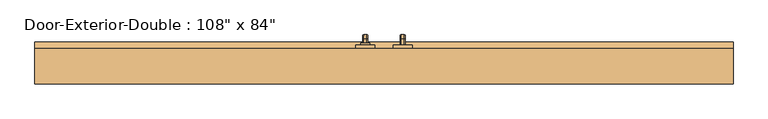
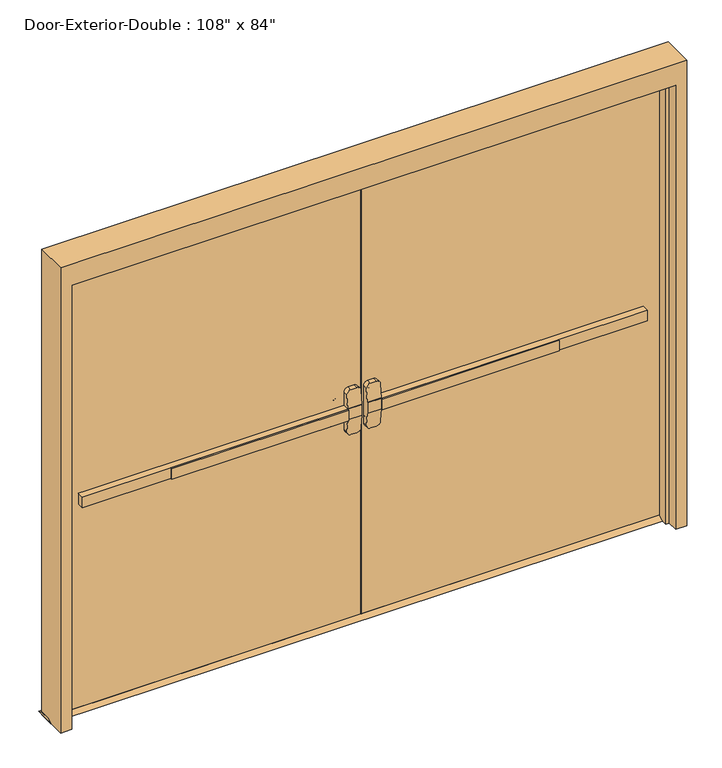
"""IFC4 building model written with IfcOpenShell, lengths in millimetres: door geometry."""

from ifc_helpers import new_model, si_unit, point, frame, frame_2d, origin, place, context, project, spatial, polyline, circle_curve, ellipse_curve, trimmed, segment, composite_curve, outline, extrude, faceted_brep, source, transform, mapped, element, save
from ifc_brep_helpers import plane_surface, cylinder_surface, revolved_surface, advanced_brep


def door_b5c84c7e(model_context):
    return source(origin(), model_context, "Body", "SolidModel", [
        extrude(outline(polyline([(-880.5333333, 0.0), (-880.5333333, 6.35), (-76.2, 6.35), (-76.2, 0.0), (-880.5333333, 0.0)])), frame((0.0, 0.0, 990.6), z_axis=(0.0, 0.0, 1.0), x_axis=(1.0, 0.0, 0.0)), (0.0, 0.0, 1.0), 50.8),
        advanced_brep(
        [(-12.7, 6.35, 1041.4), (-76.2, 6.35, 1041.4), (-1282.7, 6.35, 1041.4), (-1282.7, 6.35, 990.6), (-76.2, 6.35, 990.6), (-12.7, 6.35, 990.6), (-1282.7, 38.1, 1041.4), (-76.2, 38.1, 1041.4), (-76.2, 38.1, 1104.9), (-57.15, 38.1, 1123.95), (-31.75, 38.1, 1123.95), (-12.7, 38.1, 1104.9), (-12.7, 38.1, 927.1), (-31.75, 38.1, 908.05), (-57.15, 38.1, 908.05), (-76.2, 38.1, 927.1), (-76.2, 38.1, 990.6), (-1282.7, 38.1, 990.6), (-12.7, 9.5252467, 1041.4), (-76.2, 9.5252467, 1041.4), (-12.7, 9.5252467, 990.6), (-12.7, 14.5354269, 927.1), (-12.7, 14.5354269, 1104.9), (-76.2, 9.5252467, 990.6), (-76.2, 14.5354269, 1104.9), (-76.2, 14.5354269, 927.1), (-57.15, 16.038481, 1123.95), (-31.75, 16.038481, 1123.95), (-31.75, 16.038481, 908.05), (-57.15, 16.038481, 908.05)],
        [
            (0, 1),
            (1, 2),
            (2, 3),
            (3, 4),
            (4, 5),
            (5, 0),
            (6, 7),
            (7, 8),
            (8, 9, circle_curve(frame((-57.15, 38.1, 1104.9), z_axis=(0.0, 1.0, 0.0), x_axis=(-1.0, 0.0, 0.0)), 19.05)),
            (9, 10),
            (10, 11, circle_curve(frame((-31.75, 38.1, 1104.9), z_axis=(0.0, 1.0, 0.0), x_axis=(-1.0, 0.0, 0.0)), 19.05)),
            (11, 12),
            (12, 13, circle_curve(frame((-31.75, 38.1, 927.1), z_axis=(0.0, 1.0, 0.0), x_axis=(-1.0, 0.0, 0.0)), 19.05)),
            (13, 14),
            (14, 15, circle_curve(frame((-57.15, 38.1, 927.1), z_axis=(0.0, 1.0, 0.0), x_axis=(-1.0, 0.0, 0.0)), 19.05)),
            (15, 16),
            (16, 17),
            (17, 6),
            (0, 18),
            (18, 19),
            (19, 7),
            (6, 2),
            (5, 20),
            (20, 21),
            (21, 12),
            (11, 22),
            (22, 18),
            (16, 23),
            (23, 20),
            (3, 17),
            (19, 24),
            (24, 8),
            (15, 25),
            (25, 23),
            (9, 26),
            (26, 27),
            (27, 10),
            (13, 28),
            (28, 29),
            (29, 14),
            (29, 25, ellipse_curve(frame((-57.15, 14.5354269, 927.1), z_axis=(0.0, 0.9969018152893365, 0.07865602756830282), x_axis=(0.0, -0.07865602756830208, 0.9969018152893365)), 19.1092038, 19.05)),
            (24, 26, ellipse_curve(frame((-57.15, 14.5354269, 1104.9), z_axis=(0.0, 0.9969018152893376, -0.07865602756828934), x_axis=(0.0, -0.078656027568288, -0.9969018152893377)), 19.1092038, 19.05)),
            (27, 22, ellipse_curve(frame((-31.75, 14.5354269, 1104.9), z_axis=(0.0, 0.9969018152893376, -0.07865602756828934), x_axis=(0.0, -0.078656027568288, -0.9969018152893377)), 19.1092038, 19.05)),
            (21, 28, ellipse_curve(frame((-31.75, 14.5354269, 927.1), z_axis=(0.0, 0.9969018152893365, 0.07865602756830282), x_axis=(0.0, -0.07865602756830208, 0.9969018152893365)), 19.1092038, 19.05)),
        ],
        [
            plane_surface(frame((-12.7, 6.35, 1041.4), z_axis=(0.0, -1.0, 0.0), x_axis=(1.0, 0.0, 0.0))),
            plane_surface(frame((-12.7, 38.1, 1041.4), z_axis=(0.0, 1.0, 0.0), x_axis=(-1.0, 0.0, 0.0))),
            plane_surface(frame((-1282.7, 6.35, 1041.4), z_axis=(0.0, 0.0, 1.0), x_axis=(0.0, 1.0, 0.0))),
            plane_surface(frame((-12.7, 6.35, 1041.4), z_axis=(1.0, 0.0, 0.0), x_axis=(0.0, 1.0, 0.0))),
            plane_surface(frame((-12.7, 6.35, 990.6), z_axis=(0.0, 0.0, -1.0), x_axis=(0.0, 1.0, 0.0))),
            plane_surface(frame((-1282.7, 6.35, 990.6), z_axis=(-1.0, 0.0, 0.0), x_axis=(0.0, 1.0, 0.0))),
            plane_surface(frame((-76.2, 9.5252467, 927.1), z_axis=(-1.0, 0.0, 0.0), x_axis=(0.0, 1.0, 0.0))),
            plane_surface(frame((-57.15, 9.5252467, 1123.95), z_axis=(0.0, 0.0, 1.0), x_axis=(0.0, 1.0, 0.0))),
            plane_surface(frame((-31.75, 9.5252467, 908.05), z_axis=(0.0, 0.0, -1.0), x_axis=(0.0, 1.0, 0.0))),
            cylinder_surface(frame((-57.15, 38.1, 927.1), z_axis=(0.0, -1.0, 0.0), x_axis=(-1.0, 0.0, 0.0)), 19.05),
            cylinder_surface(frame((-57.15, 38.1, 1104.9), z_axis=(0.0, -1.0, 0.0), x_axis=(-1.0, 0.0, 0.0)), 19.05),
            cylinder_surface(frame((-31.75, 38.1, 1104.9), z_axis=(0.0, -1.0, 0.0), x_axis=(-1.0, 0.0, 0.0)), 19.05),
            cylinder_surface(frame((-31.75, 38.1, 927.1), z_axis=(0.0, -1.0, 0.0), x_axis=(-1.0, 0.0, 0.0)), 19.05),
            plane_surface(frame((-76.2, 9.5252467, 1041.4), z_axis=(0.0, -0.9969018152893376, 0.07865602756828934), x_axis=(1.0, 0.0, 0.0))),
            plane_surface(frame((-76.2, 16.038481, 908.05), z_axis=(0.0, -0.9969018152893365, -0.07865602756830282), x_axis=(1.0, 0.0, 0.0))),
        ],
        [
            (0, [[1, 2, 3, 4, 5, 6]]),
            (1, [[7, 8, 9, 10, 11, 12, 13, 14, 15, 16, 17, 18]]),
            (2, [[-2, -1, 19, 20, 21, -7, 22]]),
            (3, [[23, 24, 25, -12, 26, 27, -19, -6]]),
            (4, [[-17, 28, 29, -23, -5, -4, 30]]),
            (5, [[-22, -18, -30, -3]]),
            (6, [[-21, 31, 32, -8]]),
            (6, [[33, 34, -28, -16]]),
            (7, [[35, 36, 37, -10]]),
            (8, [[38, 39, 40, -14]]),
            (9, [[-40, 41, -33, -15]]),
            (10, [[-32, 42, -35, -9]]),
            (11, [[-37, 43, -26, -11]]),
            (12, [[-25, 44, -38, -13]]),
            (13, [[-27, -43, -36, -42, -31, -20]]),
            (14, [[-29, -34, -41, -39, -44, -24]]),
        ],
    ),
        extrude(outline(polyline([(82.55, 12.7), (107.95, 0.0), (12.7, 0.0), (38.1, 12.7), (82.55, 12.7)])), frame((-1422.4, 0.0, 0.0), z_axis=(1.0, 0.0, 0.0), x_axis=(0.0, 1.0, 0.0)), (0.0, 0.0, 1.0), 2844.8),
        extrude(outline(polyline([(880.5333333, 0.0), (76.2, 0.0), (76.2, 6.35), (880.5333333, 6.35), (880.5333333, 0.0)])), frame((0.0, 0.0, 990.6), z_axis=(0.0, 0.0, 1.0), x_axis=(1.0, 0.0, 0.0)), (0.0, 0.0, 1.0), 50.8),
        advanced_brep(
        [(12.7, 6.35, 1041.4), (12.7, 6.35, 990.6), (76.2, 6.35, 990.6), (1282.7, 6.35, 990.6), (1282.7, 6.35, 1041.4), (76.2, 6.35, 1041.4), (1282.7, 38.1, 1041.4), (1282.7, 38.1, 990.6), (76.2, 38.1, 990.6), (76.2, 38.1, 927.1), (57.15, 38.1, 908.05), (31.75, 38.1, 908.05), (12.7, 38.1, 927.1), (12.7, 38.1, 1104.9), (31.75, 38.1, 1123.95), (57.15, 38.1, 1123.95), (76.2, 38.1, 1104.9), (76.2, 38.1, 1041.4), (76.2, 9.5252467, 1041.4), (12.7, 9.5252467, 1041.4), (12.7, 14.5354269, 1104.9), (12.7, 14.5354269, 927.1), (12.7, 9.5252467, 990.6), (76.2, 9.5252467, 990.6), (76.2, 14.5354269, 927.1), (76.2, 14.5354269, 1104.9), (31.75, 16.038481, 1123.95), (57.15, 16.038481, 1123.95), (57.15, 16.038481, 908.05), (31.75, 16.038481, 908.05)],
        [
            (0, 1),
            (1, 2),
            (2, 3),
            (3, 4),
            (4, 5),
            (5, 0),
            (6, 7),
            (7, 8),
            (8, 9),
            (9, 10, circle_curve(frame((57.15, 38.1, 927.1), z_axis=(0.0, 1.0, 0.0), x_axis=(1.0, 0.0, 0.0)), 19.05)),
            (10, 11),
            (11, 12, circle_curve(frame((31.75, 38.1, 927.1), z_axis=(0.0, 1.0, 0.0), x_axis=(1.0, 0.0, 0.0)), 19.05)),
            (12, 13),
            (13, 14, circle_curve(frame((31.75, 38.1, 1104.9), z_axis=(0.0, 1.0, 0.0), x_axis=(1.0, 0.0, 0.0)), 19.05)),
            (14, 15),
            (15, 16, circle_curve(frame((57.15, 38.1, 1104.9), z_axis=(0.0, 1.0, 0.0), x_axis=(1.0, 0.0, 0.0)), 19.05)),
            (16, 17),
            (17, 6),
            (4, 6),
            (17, 18),
            (18, 19),
            (19, 0),
            (19, 20),
            (20, 13),
            (12, 21),
            (21, 22),
            (22, 1),
            (7, 3),
            (22, 23),
            (23, 8),
            (23, 24),
            (24, 9),
            (16, 25),
            (25, 18),
            (14, 26),
            (26, 27),
            (27, 15),
            (10, 28),
            (28, 29),
            (29, 11),
            (24, 28, ellipse_curve(frame((57.15, 14.5354269, 927.1), z_axis=(0.0, 0.9969018152893365, 0.07865602756830282), x_axis=(0.0, -0.07865602756830208, 0.9969018152893365)), 19.1092038, 19.05)),
            (27, 25, ellipse_curve(frame((57.15, 14.5354269, 1104.9), z_axis=(0.0, 0.9969018152893376, -0.07865602756828934), x_axis=(0.0, -0.078656027568288, -0.9969018152893377)), 19.1092038, 19.05)),
            (20, 26, ellipse_curve(frame((31.75, 14.5354269, 1104.9), z_axis=(0.0, 0.9969018152893376, -0.07865602756828934), x_axis=(0.0, -0.078656027568288, -0.9969018152893377)), 19.1092038, 19.05)),
            (29, 21, ellipse_curve(frame((31.75, 14.5354269, 927.1), z_axis=(0.0, 0.9969018152893365, 0.07865602756830282), x_axis=(0.0, -0.07865602756830208, 0.9969018152893365)), 19.1092038, 19.05)),
        ],
        [
            plane_surface(frame((12.7, 6.35, 1041.4), z_axis=(0.0, -1.0, 0.0), x_axis=(-1.0, 0.0, 0.0))),
            plane_surface(frame((12.7, 38.1, 1041.4), z_axis=(0.0, 1.0, 0.0), x_axis=(1.0, 0.0, 0.0))),
            plane_surface(frame((1282.7, 6.35, 1041.4), z_axis=(0.0, 0.0, 1.0), x_axis=(0.0, 1.0, 0.0))),
            plane_surface(frame((12.7, 6.35, 1041.4), z_axis=(-1.0, 0.0, 0.0), x_axis=(0.0, 1.0, 0.0))),
            plane_surface(frame((12.7, 6.35, 990.6), z_axis=(0.0, 0.0, -1.0), x_axis=(0.0, 1.0, 0.0))),
            plane_surface(frame((1282.7, 6.35, 990.6), z_axis=(1.0, 0.0, 0.0), x_axis=(0.0, 1.0, 0.0))),
            plane_surface(frame((76.2, 9.5252467, 927.1), z_axis=(1.0, 0.0, 0.0), x_axis=(0.0, 1.0, 0.0))),
            plane_surface(frame((57.15, 9.5252467, 1123.95), z_axis=(0.0, 0.0, 1.0), x_axis=(0.0, 1.0, 0.0))),
            plane_surface(frame((31.75, 9.5252467, 908.05), z_axis=(0.0, 0.0, -1.0), x_axis=(0.0, 1.0, 0.0))),
            cylinder_surface(frame((57.15, 38.1, 927.1), z_axis=(0.0, -1.0, 0.0), x_axis=(1.0, 0.0, 0.0)), 19.05),
            cylinder_surface(frame((57.15, 38.1, 1104.9), z_axis=(0.0, -1.0, 0.0), x_axis=(1.0, 0.0, 0.0)), 19.05),
            cylinder_surface(frame((31.75, 38.1, 1104.9), z_axis=(0.0, -1.0, 0.0), x_axis=(1.0, 0.0, 0.0)), 19.05),
            cylinder_surface(frame((31.75, 38.1, 927.1), z_axis=(0.0, -1.0, 0.0), x_axis=(1.0, 0.0, 0.0)), 19.05),
            plane_surface(frame((76.2, 9.5252467, 1041.4), z_axis=(0.0, -0.9969018152893376, 0.07865602756828934), x_axis=(-1.0, 0.0, 0.0))),
            plane_surface(frame((76.2, 16.038481, 908.05), z_axis=(0.0, -0.9969018152893365, -0.07865602756830282), x_axis=(-1.0, 0.0, 0.0))),
        ],
        [
            (0, [[1, 2, 3, 4, 5, 6]]),
            (1, [[7, 8, 9, 10, 11, 12, 13, 14, 15, 16, 17, 18]]),
            (2, [[19, -18, 20, 21, 22, -6, -5]]),
            (3, [[-1, -22, 23, 24, -13, 25, 26, 27]]),
            (4, [[28, -3, -2, -27, 29, 30, -8]]),
            (5, [[-4, -28, -7, -19]]),
            (6, [[-9, -30, 31, 32]]),
            (6, [[-17, 33, 34, -20]]),
            (7, [[-15, 35, 36, 37]]),
            (8, [[-11, 38, 39, 40]]),
            (9, [[-10, -32, 41, -38]]),
            (10, [[-16, -37, 42, -33]]),
            (11, [[-14, -24, 43, -35]]),
            (12, [[-12, -40, 44, -25]]),
            (13, [[-21, -34, -42, -36, -43, -23]]),
            (14, [[-26, -44, -39, -41, -31, -29]]),
        ],
    ),
        advanced_brep(
        [(66.2, 95.25, 1017.190625), (66.2, 95.25, 1014.809375), (69.771875, 95.25, 1011.2375), (82.6284594, 95.25, 1011.2375), (86.2, 95.25, 1014.8090406), (86.2, 95.25, 1017.190625), (82.628125, 95.25, 1020.7625), (69.771875, 95.25, 1020.7625), (66.2, 95.25, 887.809375), (69.771875, 95.25, 884.2375), (82.628125, 95.25, 884.2375), (86.2, 95.25, 887.809375), (86.2, 95.25, 890.1909594), (82.6284594, 95.25, 893.7625), (69.771875, 95.25, 893.7625), (66.2, 95.25, 890.190625), (66.2, 120.65, 1017.190625), (66.2, 134.540625, 1003.3), (66.2, 134.540625, 901.7), (66.2, 120.65, 887.809375), (66.2, 120.65, 890.190625), (66.2, 132.159375, 901.7), (66.2, 132.159375, 1003.3), (66.2, 120.65, 1014.809375), (69.771875, 120.65, 1011.2375), (82.6284594, 120.65, 1011.2375), (86.2, 120.65, 1014.8090406), (86.2, 132.1590406, 1003.3), (86.2, 132.1590406, 901.7), (86.2, 120.65, 890.1909594), (86.2, 120.65, 887.809375), (86.2, 134.540625, 901.7), (86.2, 134.540625, 1003.3), (86.2, 120.65, 1017.190625), (82.628125, 120.65, 1020.7625), (69.771875, 120.65, 1020.7625), (69.771875, 128.5875, 1003.3), (82.6284594, 128.5875, 1003.3), (82.628125, 138.1125, 1003.3), (69.771875, 138.1125, 1003.3), (69.771875, 128.5875, 901.7), (82.6284594, 128.5875, 901.7), (82.628125, 138.1125, 901.7), (69.771875, 138.1125, 901.7), (69.771875, 120.65, 893.7625), (82.6284594, 120.65, 893.7625), (82.628125, 120.65, 884.2375), (69.771875, 120.65, 884.2375)],
        [
            (0, 1),
            (1, 2, circle_curve(frame((69.771875, 95.25, 1014.809375), z_axis=(0.0, -1.0, 0.0), x_axis=(0.0, 0.0, 1.0)), 3.571875)),
            (2, 3),
            (3, 4, circle_curve(frame((82.6284594, 95.25, 1014.8090406), z_axis=(0.0, -1.0, 0.0), x_axis=(0.0, 0.0, 1.0)), 3.5715406)),
            (4, 5),
            (5, 6, circle_curve(frame((82.628125, 95.25, 1017.190625), z_axis=(0.0, -1.0, 0.0), x_axis=(0.0, 0.0, 1.0)), 3.571875)),
            (6, 7),
            (7, 0, circle_curve(frame((69.771875, 95.25, 1017.190625), z_axis=(0.0, -1.0, 0.0), x_axis=(0.0, 0.0, 1.0)), 3.571875)),
            (8, 9, circle_curve(frame((69.771875, 95.25, 887.809375), z_axis=(0.0, -1.0, 0.0), x_axis=(0.0, 0.0, -1.0)), 3.571875)),
            (9, 10),
            (10, 11, circle_curve(frame((82.628125, 95.25, 887.809375), z_axis=(0.0, -1.0, 0.0), x_axis=(0.0, 0.0, -1.0)), 3.571875)),
            (11, 12),
            (12, 13, circle_curve(frame((82.6284594, 95.25, 890.1909594), z_axis=(0.0, -1.0, 0.0), x_axis=(0.0, 0.0, -1.0)), 3.5715406)),
            (13, 14),
            (14, 15, circle_curve(frame((69.771875, 95.25, 890.190625), z_axis=(0.0, -1.0, 0.0), x_axis=(0.0, 0.0, -1.0)), 3.571875)),
            (15, 8),
            (0, 16),
            (16, 17, circle_curve(frame((66.2, 120.65, 1003.3), z_axis=(-1.0, 0.0, 0.0), x_axis=(0.0, 0.0, 1.0)), 13.890625)),
            (17, 18),
            (18, 19, circle_curve(frame((66.2, 120.65, 901.7), z_axis=(-1.0, 0.0, 0.0), x_axis=(0.0, 1.0, 0.0)), 13.890625)),
            (19, 8),
            (15, 20),
            (20, 21, circle_curve(frame((66.2, 120.65, 901.7), z_axis=(1.0, 0.0, 0.0), x_axis=(0.0, 1.0, 0.0)), 11.509375)),
            (21, 22),
            (22, 23, circle_curve(frame((66.2, 120.65, 1003.3), z_axis=(1.0, 0.0, 0.0), x_axis=(0.0, 0.0, 1.0)), 11.509375)),
            (23, 1),
            (23, 24, circle_curve(frame((69.771875, 120.65, 1014.809375), z_axis=(0.0, -1.0, 0.0), x_axis=(0.0, 0.0, 1.0)), 3.571875)),
            (24, 2),
            (24, 25),
            (25, 3),
            (25, 26, circle_curve(frame((82.6284594, 120.65, 1014.8090406), z_axis=(0.0, -1.0, 0.0), x_axis=(0.0, 0.0, 1.0)), 3.5715406)),
            (26, 4),
            (26, 27, circle_curve(frame((86.2, 120.65, 1003.3), z_axis=(-1.0, 0.0, 0.0), x_axis=(0.0, 0.0, 1.0)), 11.5090406)),
            (27, 28),
            (28, 29, circle_curve(frame((86.2, 120.65, 901.7), z_axis=(-1.0, 0.0, 0.0), x_axis=(0.0, 1.0, 0.0)), 11.5090406)),
            (29, 12),
            (11, 30),
            (30, 31, circle_curve(frame((86.2, 120.65, 901.7), z_axis=(1.0, 0.0, 0.0), x_axis=(0.0, 1.0, 0.0)), 13.890625)),
            (31, 32),
            (32, 33, circle_curve(frame((86.2, 120.65, 1003.3), z_axis=(1.0, 0.0, 0.0), x_axis=(0.0, 0.0, 1.0)), 13.890625)),
            (33, 5),
            (33, 34, circle_curve(frame((82.628125, 120.65, 1017.190625), z_axis=(0.0, -1.0, 0.0), x_axis=(0.0, 0.0, 1.0)), 3.571875)),
            (34, 6),
            (34, 35),
            (35, 7),
            (35, 16, circle_curve(frame((69.771875, 120.65, 1017.190625), z_axis=(0.0, -1.0, 0.0), x_axis=(0.0, 0.0, 1.0)), 3.571875)),
            (36, 24, circle_curve(frame((69.771875, 120.65, 1003.3), z_axis=(1.0, 0.0, 0.0), x_axis=(0.0, 0.0, 1.0)), 7.9375)),
            (22, 36, circle_curve(frame((69.771875, 132.159375, 1003.3), z_axis=(0.0, 0.0, 1.0), x_axis=(0.0, 1.0, 0.0)), 3.571875)),
            (37, 25, circle_curve(frame((82.6284594, 120.65, 1003.3), z_axis=(1.0, 0.0, 0.0), x_axis=(0.0, 0.0, 1.0)), 7.9375)),
            (36, 37),
            (37, 27, circle_curve(frame((82.6284594, 132.1590406, 1003.3), z_axis=(0.0, 0.0, 1.0), x_axis=(0.0, 1.0, 0.0)), 3.5715406)),
            (38, 34, circle_curve(frame((82.628125, 120.65, 1003.3), z_axis=(1.0, 0.0, 0.0), x_axis=(0.0, 0.0, 1.0)), 17.4625)),
            (32, 38, circle_curve(frame((82.628125, 134.540625, 1003.3), z_axis=(0.0, 0.0, 1.0), x_axis=(0.0, 1.0, 0.0)), 3.571875)),
            (39, 35, circle_curve(frame((69.771875, 120.65, 1003.3), z_axis=(1.0, 0.0, 0.0), x_axis=(0.0, 0.0, 1.0)), 17.4625)),
            (38, 39),
            (39, 17, circle_curve(frame((69.771875, 134.540625, 1003.3), z_axis=(0.0, 0.0, 1.0), x_axis=(0.0, 1.0, 0.0)), 3.571875)),
            (21, 40, circle_curve(frame((69.771875, 132.159375, 901.7), z_axis=(0.0, 0.0, 1.0), x_axis=(0.0, 1.0, 0.0)), 3.571875)),
            (40, 36),
            (40, 41),
            (41, 37),
            (41, 28, circle_curve(frame((82.6284594, 132.1590406, 901.7), z_axis=(0.0, 0.0, 1.0), x_axis=(0.0, 1.0, 0.0)), 3.5715406)),
            (31, 42, circle_curve(frame((82.628125, 134.540625, 901.7), z_axis=(0.0, 0.0, 1.0), x_axis=(0.0, 1.0, 0.0)), 3.571875)),
            (42, 38),
            (42, 43),
            (43, 39),
            (43, 18, circle_curve(frame((69.771875, 134.540625, 901.7), z_axis=(0.0, 0.0, 1.0), x_axis=(0.0, 1.0, 0.0)), 3.571875)),
            (44, 40, circle_curve(frame((69.771875, 120.65, 901.7), z_axis=(1.0, 0.0, 0.0), x_axis=(0.0, 1.0, 0.0)), 7.9375)),
            (20, 44, circle_curve(frame((69.771875, 120.65, 890.190625), z_axis=(0.0, 1.0, 0.0), x_axis=(0.0, 0.0, -1.0)), 3.571875)),
            (45, 41, circle_curve(frame((82.6284594, 120.65, 901.7), z_axis=(1.0, 0.0, 0.0), x_axis=(0.0, 1.0, 0.0)), 7.9375)),
            (44, 45),
            (45, 29, circle_curve(frame((82.6284594, 120.65, 890.1909594), z_axis=(0.0, 1.0, 0.0), x_axis=(0.0, 0.0, -1.0)), 3.5715406)),
            (46, 42, circle_curve(frame((82.628125, 120.65, 901.7), z_axis=(1.0, 0.0, 0.0), x_axis=(0.0, 1.0, 0.0)), 17.4625)),
            (30, 46, circle_curve(frame((82.628125, 120.65, 887.809375), z_axis=(0.0, 1.0, 0.0), x_axis=(0.0, 0.0, -1.0)), 3.571875)),
            (47, 43, circle_curve(frame((69.771875, 120.65, 901.7), z_axis=(1.0, 0.0, 0.0), x_axis=(0.0, 1.0, 0.0)), 17.4625)),
            (46, 47),
            (47, 19, circle_curve(frame((69.771875, 120.65, 887.809375), z_axis=(0.0, 1.0, 0.0), x_axis=(0.0, 0.0, -1.0)), 3.571875)),
            (14, 44),
            (13, 45),
            (10, 46),
            (9, 47),
        ],
        [
            plane_surface(frame((76.2, 95.25, 1016.0), z_axis=(0.0, -1.0, 0.0), x_axis=(1.0, 0.0, 0.0))),
            plane_surface(frame((76.2, 95.25, 889.0), z_axis=(0.0, -1.0, 0.0), x_axis=(1.0, 0.0, 0.0))),
            plane_surface(frame((66.2, 95.25, 1017.190625), z_axis=(-1.0, 0.0, 0.0), x_axis=(0.0, 1.0, 0.0))),
            cylinder_surface(frame((69.771875, 95.25, 1014.809375), z_axis=(0.0, -1.0, 0.0), x_axis=(0.0, 0.0, 1.0)), 3.571875),
            plane_surface(frame((69.771875, 95.25, 1011.2375), z_axis=(0.0, 0.0, -1.0), x_axis=(0.0, 1.0, 0.0))),
            cylinder_surface(frame((82.6284594, 95.25, 1014.8090406), z_axis=(0.0, -1.0, 0.0), x_axis=(0.0, 0.0, 1.0)), 3.5715406),
            plane_surface(frame((86.2, 95.25, 1014.8090406), z_axis=(1.0, 0.0, 0.0), x_axis=(0.0, 1.0, 0.0))),
            cylinder_surface(frame((82.628125, 95.25, 1017.190625), z_axis=(0.0, -1.0, 0.0), x_axis=(0.0, 0.0, 1.0)), 3.571875),
            plane_surface(frame((82.628125, 95.25, 1020.7625), z_axis=(0.0, 0.0, 1.0), x_axis=(0.0, 1.0, 0.0))),
            cylinder_surface(frame((69.771875, 95.25, 1017.190625), z_axis=(0.0, -1.0, 0.0), x_axis=(0.0, 0.0, 1.0)), 3.571875),
            revolved_surface(trimmed(ellipse_curve(frame((69.771875, 120.65, 1014.809375), z_axis=(0.0, -1.0, 0.0), x_axis=(0.0, 0.0, 1.0)), 3.571875, 3.571875), [point((66.2, 120.65, 1014.809375))], [point((69.771875, 120.65, 1011.2375))], True, "CARTESIAN"), (76.2, 120.65, 1003.3), (-1.0, 0.0, 0.0)),
            revolved_surface(polyline([(69.771875, 120.65, 1011.2375), (82.6284594, 120.65, 1011.2375)]), (76.2, 120.65, 1003.3), (-1.0, 0.0, 0.0)),
            revolved_surface(trimmed(ellipse_curve(frame((82.6284594, 120.65, 1014.8090406), z_axis=(0.0, -1.0, 0.0), x_axis=(0.0, 0.0, 1.0)), 3.5715406, 3.5715406), [point((82.6284594, 120.65, 1011.2375))], [point((86.2, 120.65, 1014.8090406))], True, "CARTESIAN"), (76.2, 120.65, 1003.3), (-1.0, 0.0, 0.0)),
            revolved_surface(trimmed(ellipse_curve(frame((82.628125, 120.65, 1017.190625), z_axis=(0.0, -1.0, 0.0), x_axis=(0.0, 0.0, 1.0)), 3.571875, 3.571875), [point((86.2, 120.65, 1017.190625))], [point((82.628125, 120.65, 1020.7625))], True, "CARTESIAN"), (76.2, 120.65, 1003.3), (-1.0, 0.0, 0.0)),
            cylinder_surface(frame((76.2, 120.65, 1003.3), z_axis=(-1.0, 0.0, 0.0), x_axis=(0.0, 0.0, 1.0)), 17.4625),
            revolved_surface(trimmed(ellipse_curve(frame((69.771875, 120.65, 1017.190625), z_axis=(0.0, -1.0, 0.0), x_axis=(0.0, 0.0, 1.0)), 3.571875, 3.571875), [point((69.771875, 120.65, 1020.7625))], [point((66.2, 120.65, 1017.190625))], True, "CARTESIAN"), (76.2, 120.65, 1003.3), (-1.0, 0.0, 0.0)),
            cylinder_surface(frame((69.771875, 132.159375, 1003.3), z_axis=(0.0, 0.0, 1.0), x_axis=(0.0, 1.0, 0.0)), 3.571875),
            plane_surface(frame((69.771875, 128.5875, 1003.3), z_axis=(0.0, -1.0, 0.0), x_axis=(0.0, 0.0, -1.0))),
            cylinder_surface(frame((82.6284594, 132.1590406, 1003.3), z_axis=(0.0, 0.0, 1.0), x_axis=(0.0, 1.0, 0.0)), 3.5715406),
            cylinder_surface(frame((82.628125, 134.540625, 1003.3), z_axis=(0.0, 0.0, 1.0), x_axis=(0.0, 1.0, 0.0)), 3.571875),
            plane_surface(frame((82.628125, 138.1125, 1003.3), z_axis=(0.0, 1.0, 0.0), x_axis=(0.0, 0.0, -1.0))),
            cylinder_surface(frame((69.771875, 134.540625, 1003.3), z_axis=(0.0, 0.0, 1.0), x_axis=(0.0, 1.0, 0.0)), 3.571875),
            revolved_surface(trimmed(ellipse_curve(frame((69.771875, 132.159375, 901.7), z_axis=(0.0, 0.0, 1.0), x_axis=(0.0, 1.0, 0.0)), 3.571875, 3.571875), [point((66.2, 132.159375, 901.7))], [point((69.771875, 128.5875, 901.7))], True, "CARTESIAN"), (76.2, 120.65, 901.7), (-1.0, 0.0, 0.0)),
            revolved_surface(polyline([(69.771875, 128.5875, 901.7), (82.6284594, 128.5875, 901.7)]), (76.2, 120.65, 901.7), (-1.0, 0.0, 0.0)),
            revolved_surface(trimmed(ellipse_curve(frame((82.6284594, 132.1590406, 901.7), z_axis=(0.0, 0.0, 1.0), x_axis=(0.0, 1.0, 0.0)), 3.5715406, 3.5715406), [point((82.6284594, 128.5875, 901.7))], [point((86.2, 132.1590406, 901.7))], True, "CARTESIAN"), (76.2, 120.65, 901.7), (-1.0, 0.0, 0.0)),
            revolved_surface(trimmed(ellipse_curve(frame((82.628125, 134.540625, 901.7), z_axis=(0.0, 0.0, 1.0), x_axis=(0.0, 1.0, 0.0)), 3.571875, 3.571875), [point((86.2, 134.540625, 901.7))], [point((82.628125, 138.1125, 901.7))], True, "CARTESIAN"), (76.2, 120.65, 901.7), (-1.0, 0.0, 0.0)),
            cylinder_surface(frame((76.2, 120.65, 901.7), z_axis=(-1.0, 0.0, 0.0), x_axis=(0.0, 1.0, 0.0)), 17.4625),
            revolved_surface(trimmed(ellipse_curve(frame((69.771875, 134.540625, 901.7), z_axis=(0.0, 0.0, 1.0), x_axis=(0.0, 1.0, 0.0)), 3.571875, 3.571875), [point((69.771875, 138.1125, 901.7))], [point((66.2, 134.540625, 901.7))], True, "CARTESIAN"), (76.2, 120.65, 901.7), (-1.0, 0.0, 0.0)),
            cylinder_surface(frame((69.771875, 120.65, 890.190625), z_axis=(0.0, 1.0, 0.0), x_axis=(0.0, 0.0, -1.0)), 3.571875),
            plane_surface(frame((69.771875, 120.65, 893.7625), z_axis=(0.0, 0.0, 1.0), x_axis=(0.0, -1.0, 0.0))),
            cylinder_surface(frame((82.6284594, 120.65, 890.1909594), z_axis=(0.0, 1.0, 0.0), x_axis=(0.0, 0.0, -1.0)), 3.5715406),
            cylinder_surface(frame((82.628125, 120.65, 887.809375), z_axis=(0.0, 1.0, 0.0), x_axis=(0.0, 0.0, -1.0)), 3.571875),
            plane_surface(frame((82.628125, 120.65, 884.2375), z_axis=(0.0, 0.0, -1.0), x_axis=(0.0, -1.0, 0.0))),
            cylinder_surface(frame((69.771875, 120.65, 887.809375), z_axis=(0.0, 1.0, 0.0), x_axis=(0.0, 0.0, -1.0)), 3.571875),
        ],
        [
            (0, [[1, 2, 3, 4, 5, 6, 7, 8]]),
            (1, [[9, 10, 11, 12, 13, 14, 15, 16]]),
            (2, [[-1, 17, 18, 19, 20, 21, -16, 22, 23, 24, 25, 26]]),
            (3, [[-2, -26, 27, 28]]),
            (4, [[-3, -28, 29, 30]]),
            (5, [[-4, -30, 31, 32]]),
            (6, [[-5, -32, 33, 34, 35, 36, -12, 37, 38, 39, 40, 41]]),
            (7, [[-6, -41, 42, 43]]),
            (8, [[-7, -43, 44, 45]]),
            (9, [[-8, -45, 46, -17]]),
            (10, [[47, -27, -25, 48]]),
            (11, [[49, -29, -47, 50]]),
            (12, [[-33, -31, -49, 51]]),
            (13, [[52, -42, -40, 53]]),
            (14, [[54, -44, -52, 55]]),
            (15, [[-18, -46, -54, 56]]),
            (16, [[-48, -24, 57, 58]]),
            (17, [[-50, -58, 59, 60]]),
            (18, [[-51, -60, 61, -34]]),
            (19, [[-53, -39, 62, 63]]),
            (20, [[-55, -63, 64, 65]]),
            (21, [[-56, -65, 66, -19]]),
            (22, [[67, -57, -23, 68]]),
            (23, [[69, -59, -67, 70]]),
            (24, [[-35, -61, -69, 71]]),
            (25, [[72, -62, -38, 73]]),
            (26, [[74, -64, -72, 75]]),
            (27, [[-20, -66, -74, 76]]),
            (28, [[-68, -22, -15, 77]]),
            (29, [[-70, -77, -14, 78]]),
            (30, [[-71, -78, -13, -36]]),
            (31, [[-73, -37, -11, 79]]),
            (32, [[-75, -79, -10, 80]]),
            (33, [[-76, -80, -9, -21]]),
        ],
    ),
        extrude(outline(composite_curve([segment(trimmed(circle_curve(frame_2d((1113.0338574, 76.2)), 89.3016225), [point((1193.8, 114.3))], [point((1193.8, 38.1))], False, "CARTESIAN"), True, "CONTINUOUS"), segment(polyline([(1193.8, 38.1), (838.2, 38.1)]), True, "CONTINUOUS"), segment(trimmed(circle_curve(frame_2d((918.9661426, 76.2)), 89.3016225), [point((838.2, 38.1))], [point((838.2, 114.3))], False, "CARTESIAN"), True, "CONTINUOUS"), segment(polyline([(838.2, 114.3), (1193.8, 114.3)]), True, "CONTINUOUS")], self_intersect=False)), frame((0.0, 82.55, 0.0), z_axis=(0.0, 1.0, 0.0), x_axis=(0.0, 0.0, 1.0)), (0.0, 0.0, 1.0), 12.7),
        advanced_brep(
        [(-86.2, 95.25, 1017.190625), (-86.2, 95.25, 1014.809375), (-82.628125, 95.25, 1011.2375), (-69.7715406, 95.25, 1011.2375), (-66.2, 95.25, 1014.8090406), (-66.2, 95.25, 1017.190625), (-69.771875, 95.25, 1020.7625), (-82.628125, 95.25, 1020.7625), (-86.2, 95.25, 887.809375), (-82.628125, 95.25, 884.2375), (-69.771875, 95.25, 884.2375), (-66.2, 95.25, 887.809375), (-66.2, 95.25, 890.1909594), (-69.7715406, 95.25, 893.7625), (-82.628125, 95.25, 893.7625), (-86.2, 95.25, 890.190625), (-86.2, 120.65, 1017.190625), (-86.2, 134.540625, 1003.3), (-86.2, 134.540625, 901.7), (-86.2, 120.65, 887.809375), (-86.2, 120.65, 890.190625), (-86.2, 132.159375, 901.7), (-86.2, 132.159375, 1003.3), (-86.2, 120.65, 1014.809375), (-82.628125, 120.65, 1011.2375), (-69.7715406, 120.65, 1011.2375), (-66.2, 120.65, 1014.8090406), (-66.2, 132.1590406, 1003.3), (-66.2, 132.1590406, 901.7), (-66.2, 120.65, 890.1909594), (-66.2, 120.65, 887.809375), (-66.2, 134.540625, 901.7), (-66.2, 134.540625, 1003.3), (-66.2, 120.65, 1017.190625), (-69.771875, 120.65, 1020.7625), (-82.628125, 120.65, 1020.7625), (-82.628125, 128.5875, 1003.3), (-69.7715406, 128.5875, 1003.3), (-69.771875, 138.1125, 1003.3), (-82.628125, 138.1125, 1003.3), (-82.628125, 128.5875, 901.7), (-69.7715406, 128.5875, 901.7), (-69.771875, 138.1125, 901.7), (-82.628125, 138.1125, 901.7), (-82.628125, 120.65, 893.7625), (-69.7715406, 120.65, 893.7625), (-69.771875, 120.65, 884.2375), (-82.628125, 120.65, 884.2375)],
        [
            (0, 1),
            (1, 2, circle_curve(frame((-82.628125, 95.25, 1014.809375), z_axis=(0.0, -1.0, 0.0), x_axis=(0.0, 0.0, 1.0)), 3.571875)),
            (2, 3),
            (3, 4, circle_curve(frame((-69.7715406, 95.25, 1014.8090406), z_axis=(0.0, -1.0, 0.0), x_axis=(0.0, 0.0, 1.0)), 3.5715406)),
            (4, 5),
            (5, 6, circle_curve(frame((-69.771875, 95.25, 1017.190625), z_axis=(0.0, -1.0, 0.0), x_axis=(0.0, 0.0, 1.0)), 3.571875)),
            (6, 7),
            (7, 0, circle_curve(frame((-82.628125, 95.25, 1017.190625), z_axis=(0.0, -1.0, 0.0), x_axis=(0.0, 0.0, 1.0)), 3.571875)),
            (8, 9, circle_curve(frame((-82.628125, 95.25, 887.809375), z_axis=(0.0, -1.0, 0.0), x_axis=(0.0, 0.0, -1.0)), 3.571875)),
            (9, 10),
            (10, 11, circle_curve(frame((-69.771875, 95.25, 887.809375), z_axis=(0.0, -1.0, 0.0), x_axis=(0.0, 0.0, -1.0)), 3.571875)),
            (11, 12),
            (12, 13, circle_curve(frame((-69.7715406, 95.25, 890.1909594), z_axis=(0.0, -1.0, 0.0), x_axis=(0.0, 0.0, -1.0)), 3.5715406)),
            (13, 14),
            (14, 15, circle_curve(frame((-82.628125, 95.25, 890.190625), z_axis=(0.0, -1.0, 0.0), x_axis=(0.0, 0.0, -1.0)), 3.571875)),
            (15, 8),
            (0, 16),
            (16, 17, circle_curve(frame((-86.2, 120.65, 1003.3), z_axis=(-1.0, 0.0, 0.0), x_axis=(0.0, 0.0, 1.0)), 13.890625)),
            (17, 18),
            (18, 19, circle_curve(frame((-86.2, 120.65, 901.7), z_axis=(-1.0, 0.0, 0.0), x_axis=(0.0, 1.0, 0.0)), 13.890625)),
            (19, 8),
            (15, 20),
            (20, 21, circle_curve(frame((-86.2, 120.65, 901.7), z_axis=(1.0, 0.0, 0.0), x_axis=(0.0, 1.0, 0.0)), 11.509375)),
            (21, 22),
            (22, 23, circle_curve(frame((-86.2, 120.65, 1003.3), z_axis=(1.0, 0.0, 0.0), x_axis=(0.0, 0.0, 1.0)), 11.509375)),
            (23, 1),
            (23, 24, circle_curve(frame((-82.628125, 120.65, 1014.809375), z_axis=(0.0, -1.0, 0.0), x_axis=(0.0, 0.0, 1.0)), 3.571875)),
            (24, 2),
            (24, 25),
            (25, 3),
            (25, 26, circle_curve(frame((-69.7715406, 120.65, 1014.8090406), z_axis=(0.0, -1.0, 0.0), x_axis=(0.0, 0.0, 1.0)), 3.5715406)),
            (26, 4),
            (26, 27, circle_curve(frame((-66.2, 120.65, 1003.3), z_axis=(-1.0, 0.0, 0.0), x_axis=(0.0, 0.0, 1.0)), 11.5090406)),
            (27, 28),
            (28, 29, circle_curve(frame((-66.2, 120.65, 901.7), z_axis=(-1.0, 0.0, 0.0), x_axis=(0.0, 1.0, 0.0)), 11.5090406)),
            (29, 12),
            (11, 30),
            (30, 31, circle_curve(frame((-66.2, 120.65, 901.7), z_axis=(1.0, 0.0, 0.0), x_axis=(0.0, 1.0, 0.0)), 13.890625)),
            (31, 32),
            (32, 33, circle_curve(frame((-66.2, 120.65, 1003.3), z_axis=(1.0, 0.0, 0.0), x_axis=(0.0, 0.0, 1.0)), 13.890625)),
            (33, 5),
            (33, 34, circle_curve(frame((-69.771875, 120.65, 1017.190625), z_axis=(0.0, -1.0, 0.0), x_axis=(0.0, 0.0, 1.0)), 3.571875)),
            (34, 6),
            (34, 35),
            (35, 7),
            (35, 16, circle_curve(frame((-82.628125, 120.65, 1017.190625), z_axis=(0.0, -1.0, 0.0), x_axis=(0.0, 0.0, 1.0)), 3.571875)),
            (36, 24, circle_curve(frame((-82.628125, 120.65, 1003.3), z_axis=(1.0, 0.0, 0.0), x_axis=(0.0, 0.0, 1.0)), 7.9375)),
            (22, 36, circle_curve(frame((-82.628125, 132.159375, 1003.3), z_axis=(0.0, 0.0, 1.0), x_axis=(0.0, 1.0, 0.0)), 3.571875)),
            (37, 25, circle_curve(frame((-69.7715406, 120.65, 1003.3), z_axis=(1.0, 0.0, 0.0), x_axis=(0.0, 0.0, 1.0)), 7.9375)),
            (36, 37),
            (37, 27, circle_curve(frame((-69.7715406, 132.1590406, 1003.3), z_axis=(0.0, 0.0, 1.0), x_axis=(0.0, 1.0, 0.0)), 3.5715406)),
            (38, 34, circle_curve(frame((-69.771875, 120.65, 1003.3), z_axis=(1.0, 0.0, 0.0), x_axis=(0.0, 0.0, 1.0)), 17.4625)),
            (32, 38, circle_curve(frame((-69.771875, 134.540625, 1003.3), z_axis=(0.0, 0.0, 1.0), x_axis=(0.0, 1.0, 0.0)), 3.571875)),
            (39, 35, circle_curve(frame((-82.628125, 120.65, 1003.3), z_axis=(1.0, 0.0, 0.0), x_axis=(0.0, 0.0, 1.0)), 17.4625)),
            (38, 39),
            (39, 17, circle_curve(frame((-82.628125, 134.540625, 1003.3), z_axis=(0.0, 0.0, 1.0), x_axis=(0.0, 1.0, 0.0)), 3.571875)),
            (21, 40, circle_curve(frame((-82.628125, 132.159375, 901.7), z_axis=(0.0, 0.0, 1.0), x_axis=(0.0, 1.0, 0.0)), 3.571875)),
            (40, 36),
            (40, 41),
            (41, 37),
            (41, 28, circle_curve(frame((-69.7715406, 132.1590406, 901.7), z_axis=(0.0, 0.0, 1.0), x_axis=(0.0, 1.0, 0.0)), 3.5715406)),
            (31, 42, circle_curve(frame((-69.771875, 134.540625, 901.7), z_axis=(0.0, 0.0, 1.0), x_axis=(0.0, 1.0, 0.0)), 3.571875)),
            (42, 38),
            (42, 43),
            (43, 39),
            (43, 18, circle_curve(frame((-82.628125, 134.540625, 901.7), z_axis=(0.0, 0.0, 1.0), x_axis=(0.0, 1.0, 0.0)), 3.571875)),
            (44, 40, circle_curve(frame((-82.628125, 120.65, 901.7), z_axis=(1.0, 0.0, 0.0), x_axis=(0.0, 1.0, 0.0)), 7.9375)),
            (20, 44, circle_curve(frame((-82.628125, 120.65, 890.190625), z_axis=(0.0, 1.0, 0.0), x_axis=(0.0, 0.0, -1.0)), 3.571875)),
            (45, 41, circle_curve(frame((-69.7715406, 120.65, 901.7), z_axis=(1.0, 0.0, 0.0), x_axis=(0.0, 1.0, 0.0)), 7.9375)),
            (44, 45),
            (45, 29, circle_curve(frame((-69.7715406, 120.65, 890.1909594), z_axis=(0.0, 1.0, 0.0), x_axis=(0.0, 0.0, -1.0)), 3.5715406)),
            (46, 42, circle_curve(frame((-69.771875, 120.65, 901.7), z_axis=(1.0, 0.0, 0.0), x_axis=(0.0, 1.0, 0.0)), 17.4625)),
            (30, 46, circle_curve(frame((-69.771875, 120.65, 887.809375), z_axis=(0.0, 1.0, 0.0), x_axis=(0.0, 0.0, -1.0)), 3.571875)),
            (47, 43, circle_curve(frame((-82.628125, 120.65, 901.7), z_axis=(1.0, 0.0, 0.0), x_axis=(0.0, 1.0, 0.0)), 17.4625)),
            (46, 47),
            (47, 19, circle_curve(frame((-82.628125, 120.65, 887.809375), z_axis=(0.0, 1.0, 0.0), x_axis=(0.0, 0.0, -1.0)), 3.571875)),
            (14, 44),
            (13, 45),
            (10, 46),
            (9, 47),
        ],
        [
            plane_surface(frame((-76.2, 95.25, 1016.0), z_axis=(0.0, -1.0, 0.0), x_axis=(1.0, 0.0, 0.0))),
            plane_surface(frame((-76.2, 95.25, 889.0), z_axis=(0.0, -1.0, 0.0), x_axis=(1.0, 0.0, 0.0))),
            plane_surface(frame((-86.2, 95.25, 1017.190625), z_axis=(-1.0, 0.0, 0.0), x_axis=(0.0, 1.0, 0.0))),
            cylinder_surface(frame((-82.628125, 95.25, 1014.809375), z_axis=(0.0, -1.0, 0.0), x_axis=(0.0, 0.0, 1.0)), 3.571875),
            plane_surface(frame((-82.628125, 95.25, 1011.2375), z_axis=(0.0, 0.0, -1.0), x_axis=(0.0, 1.0, 0.0))),
            cylinder_surface(frame((-69.7715406, 95.25, 1014.8090406), z_axis=(0.0, -1.0, 0.0), x_axis=(0.0, 0.0, 1.0)), 3.5715406),
            plane_surface(frame((-66.2, 95.25, 1014.8090406), z_axis=(1.0, 0.0, 0.0), x_axis=(0.0, 1.0, 0.0))),
            cylinder_surface(frame((-69.771875, 95.25, 1017.190625), z_axis=(0.0, -1.0, 0.0), x_axis=(0.0, 0.0, 1.0)), 3.571875),
            plane_surface(frame((-69.771875, 95.25, 1020.7625), z_axis=(0.0, 0.0, 1.0), x_axis=(0.0, 1.0, 0.0))),
            cylinder_surface(frame((-82.628125, 95.25, 1017.190625), z_axis=(0.0, -1.0, 0.0), x_axis=(0.0, 0.0, 1.0)), 3.571875),
            revolved_surface(trimmed(ellipse_curve(frame((-82.628125, 120.65, 1014.809375), z_axis=(0.0, -1.0, 0.0), x_axis=(0.0, 0.0, 1.0)), 3.571875, 3.571875), [point((-86.2, 120.65, 1014.809375))], [point((-82.628125, 120.65, 1011.2375))], True, "CARTESIAN"), (-76.2, 120.65, 1003.3), (-1.0, 0.0, 0.0)),
            revolved_surface(polyline([(-82.628125, 120.65, 1011.2375), (-69.7715406, 120.65, 1011.2375)]), (-76.2, 120.65, 1003.3), (-1.0, 0.0, 0.0)),
            revolved_surface(trimmed(ellipse_curve(frame((-69.7715406, 120.65, 1014.8090406), z_axis=(0.0, -1.0, 0.0), x_axis=(0.0, 0.0, 1.0)), 3.5715406, 3.5715406), [point((-69.7715406, 120.65, 1011.2375))], [point((-66.2, 120.65, 1014.8090406))], True, "CARTESIAN"), (-76.2, 120.65, 1003.3), (-1.0, 0.0, 0.0)),
            revolved_surface(trimmed(ellipse_curve(frame((-69.771875, 120.65, 1017.190625), z_axis=(0.0, -1.0, 0.0), x_axis=(0.0, 0.0, 1.0)), 3.571875, 3.571875), [point((-66.2, 120.65, 1017.190625))], [point((-69.771875, 120.65, 1020.7625))], True, "CARTESIAN"), (-76.2, 120.65, 1003.3), (-1.0, 0.0, 0.0)),
            cylinder_surface(frame((-76.2, 120.65, 1003.3), z_axis=(-1.0, 0.0, 0.0), x_axis=(0.0, 0.0, 1.0)), 17.4625),
            revolved_surface(trimmed(ellipse_curve(frame((-82.628125, 120.65, 1017.190625), z_axis=(0.0, -1.0, 0.0), x_axis=(0.0, 0.0, 1.0)), 3.571875, 3.571875), [point((-82.628125, 120.65, 1020.7625))], [point((-86.2, 120.65, 1017.190625))], True, "CARTESIAN"), (-76.2, 120.65, 1003.3), (-1.0, 0.0, 0.0)),
            cylinder_surface(frame((-82.628125, 132.159375, 1003.3), z_axis=(0.0, 0.0, 1.0), x_axis=(0.0, 1.0, 0.0)), 3.571875),
            plane_surface(frame((-82.628125, 128.5875, 1003.3), z_axis=(0.0, -1.0, 0.0), x_axis=(0.0, 0.0, -1.0))),
            cylinder_surface(frame((-69.7715406, 132.1590406, 1003.3), z_axis=(0.0, 0.0, 1.0), x_axis=(0.0, 1.0, 0.0)), 3.5715406),
            cylinder_surface(frame((-69.771875, 134.540625, 1003.3), z_axis=(0.0, 0.0, 1.0), x_axis=(0.0, 1.0, 0.0)), 3.571875),
            plane_surface(frame((-69.771875, 138.1125, 1003.3), z_axis=(0.0, 1.0, 0.0), x_axis=(0.0, 0.0, -1.0))),
            cylinder_surface(frame((-82.628125, 134.540625, 1003.3), z_axis=(0.0, 0.0, 1.0), x_axis=(0.0, 1.0, 0.0)), 3.571875),
            revolved_surface(trimmed(ellipse_curve(frame((-82.628125, 132.159375, 901.7), z_axis=(0.0, 0.0, 1.0), x_axis=(0.0, 1.0, 0.0)), 3.571875, 3.571875), [point((-86.2, 132.159375, 901.7))], [point((-82.628125, 128.5875, 901.7))], True, "CARTESIAN"), (-76.2, 120.65, 901.7), (-1.0, 0.0, 0.0)),
            revolved_surface(polyline([(-82.628125, 128.5875, 901.7), (-69.7715406, 128.5875, 901.7)]), (-76.2, 120.65, 901.7), (-1.0, 0.0, 0.0)),
            revolved_surface(trimmed(ellipse_curve(frame((-69.7715406, 132.1590406, 901.7), z_axis=(0.0, 0.0, 1.0), x_axis=(0.0, 1.0, 0.0)), 3.5715406, 3.5715406), [point((-69.7715406, 128.5875, 901.7))], [point((-66.2, 132.1590406, 901.7))], True, "CARTESIAN"), (-76.2, 120.65, 901.7), (-1.0, 0.0, 0.0)),
            revolved_surface(trimmed(ellipse_curve(frame((-69.771875, 134.540625, 901.7), z_axis=(0.0, 0.0, 1.0), x_axis=(0.0, 1.0, 0.0)), 3.571875, 3.571875), [point((-66.2, 134.540625, 901.7))], [point((-69.771875, 138.1125, 901.7))], True, "CARTESIAN"), (-76.2, 120.65, 901.7), (-1.0, 0.0, 0.0)),
            cylinder_surface(frame((-76.2, 120.65, 901.7), z_axis=(-1.0, 0.0, 0.0), x_axis=(0.0, 1.0, 0.0)), 17.4625),
            revolved_surface(trimmed(ellipse_curve(frame((-82.628125, 134.540625, 901.7), z_axis=(0.0, 0.0, 1.0), x_axis=(0.0, 1.0, 0.0)), 3.571875, 3.571875), [point((-82.628125, 138.1125, 901.7))], [point((-86.2, 134.540625, 901.7))], True, "CARTESIAN"), (-76.2, 120.65, 901.7), (-1.0, 0.0, 0.0)),
            cylinder_surface(frame((-82.628125, 120.65, 890.190625), z_axis=(0.0, 1.0, 0.0), x_axis=(0.0, 0.0, -1.0)), 3.571875),
            plane_surface(frame((-82.628125, 120.65, 893.7625), z_axis=(0.0, 0.0, 1.0), x_axis=(0.0, -1.0, 0.0))),
            cylinder_surface(frame((-69.7715406, 120.65, 890.1909594), z_axis=(0.0, 1.0, 0.0), x_axis=(0.0, 0.0, -1.0)), 3.5715406),
            cylinder_surface(frame((-69.771875, 120.65, 887.809375), z_axis=(0.0, 1.0, 0.0), x_axis=(0.0, 0.0, -1.0)), 3.571875),
            plane_surface(frame((-69.771875, 120.65, 884.2375), z_axis=(0.0, 0.0, -1.0), x_axis=(0.0, -1.0, 0.0))),
            cylinder_surface(frame((-82.628125, 120.65, 887.809375), z_axis=(0.0, 1.0, 0.0), x_axis=(0.0, 0.0, -1.0)), 3.571875),
        ],
        [
            (0, [[1, 2, 3, 4, 5, 6, 7, 8]]),
            (1, [[9, 10, 11, 12, 13, 14, 15, 16]]),
            (2, [[-1, 17, 18, 19, 20, 21, -16, 22, 23, 24, 25, 26]]),
            (3, [[-2, -26, 27, 28]]),
            (4, [[-3, -28, 29, 30]]),
            (5, [[-4, -30, 31, 32]]),
            (6, [[-5, -32, 33, 34, 35, 36, -12, 37, 38, 39, 40, 41]]),
            (7, [[-6, -41, 42, 43]]),
            (8, [[-7, -43, 44, 45]]),
            (9, [[-8, -45, 46, -17]]),
            (10, [[47, -27, -25, 48]]),
            (11, [[49, -29, -47, 50]]),
            (12, [[-33, -31, -49, 51]]),
            (13, [[52, -42, -40, 53]]),
            (14, [[54, -44, -52, 55]]),
            (15, [[-18, -46, -54, 56]]),
            (16, [[-48, -24, 57, 58]]),
            (17, [[-50, -58, 59, 60]]),
            (18, [[-51, -60, 61, -34]]),
            (19, [[-53, -39, 62, 63]]),
            (20, [[-55, -63, 64, 65]]),
            (21, [[-56, -65, 66, -19]]),
            (22, [[67, -57, -23, 68]]),
            (23, [[69, -59, -67, 70]]),
            (24, [[-35, -61, -69, 71]]),
            (25, [[72, -62, -38, 73]]),
            (26, [[74, -64, -72, 75]]),
            (27, [[-20, -66, -74, 76]]),
            (28, [[-68, -22, -15, 77]]),
            (29, [[-70, -77, -14, 78]]),
            (30, [[-71, -78, -13, -36]]),
            (31, [[-73, -37, -11, 79]]),
            (32, [[-75, -79, -10, 80]]),
            (33, [[-76, -80, -9, -21]]),
        ],
    ),
        extrude(outline(composite_curve([segment(trimmed(circle_curve(frame_2d((1117.6, -76.2)), 19.0), [point((1117.6, -95.2))], [point((1117.6, -57.2))], False, "CARTESIAN"), True, "CONTINUOUS"), segment(trimmed(circle_curve(frame_2d((1117.6, -76.2)), 19.0), [point((1117.6, -57.2))], [point((1117.6, -95.2))], False, "CARTESIAN"), True, "CONTINUOUS")], self_intersect=False)), frame((0.0, 95.25, 0.0), z_axis=(0.0, 1.0, 0.0), x_axis=(0.0, 0.0, 1.0)), (0.0, 0.0, 1.0), 8.73125),
        extrude(outline(composite_curve([segment(trimmed(circle_curve(frame_2d((1113.0338574, -76.2)), 89.3016225), [point((1193.8, -38.1))], [point((1193.8, -114.3))], False, "CARTESIAN"), True, "CONTINUOUS"), segment(polyline([(1193.8, -114.3), (838.2, -114.3)]), True, "CONTINUOUS"), segment(trimmed(circle_curve(frame_2d((918.9661426, -76.2)), 89.3016225), [point((838.2, -114.3))], [point((838.2, -38.1))], False, "CARTESIAN"), True, "CONTINUOUS"), segment(polyline([(838.2, -38.1), (1193.8, -38.1)]), True, "CONTINUOUS")], self_intersect=False)), frame((0.0, 82.55, 0.0), z_axis=(0.0, 1.0, 0.0), x_axis=(0.0, 0.0, 1.0)), (0.0, 0.0, 1.0), 12.7),
        faceted_brep([(1371.6, 33.3375, 0.0), (1371.6, 82.55, 0.0), (1422.4, 82.55, 0.0), (1422.4, -63.5, 0.0), (1371.6, -63.5, 0.0), (1371.6, -14.2875, 0.0), (1355.725, -14.2875, 0.0), (1355.725, 33.3375, 0.0), (1371.6, 33.3375, 2133.6), (1371.6, 82.55, 2133.6), (-1371.6, 82.55, 2133.6), (-1371.6, 82.55, 0.0), (-1422.4, 82.55, 0.0), (-1422.4, 82.55, 2235.2), (1422.4, 82.55, 2235.2), (1422.4, -63.5, 2235.2), (-1422.4, -63.5, 2235.2), (-1422.4, -63.5, 0.0), (-1371.6, -63.5, 0.0), (-1371.6, -63.5, 2133.6), (1371.6, -63.5, 2133.6), (1371.6, -14.2875, 2133.6), (-1371.6, -14.2875, 2133.6), (-1371.6, -14.2875, 0.0), (-1355.725, -14.2875, 0.0), (-1355.725, -14.2875, 2117.725), (1355.725, -14.2875, 2117.725), (1355.725, 33.3375, 2117.725), (-1355.725, 33.3375, 2117.725), (-1355.725, 33.3375, 0.0), (-1371.6, 33.3375, 0.0), (-1371.6, 33.3375, 2133.6)], [[[0, 1, 2, 3, 4, 5, 6, 7]], [[1, 0, 8, 9]], [[2, 1, 9, 10, 11, 12, 13, 14]], [[3, 2, 14, 15]], [[4, 3, 15, 16, 17, 18, 19, 20]], [[5, 4, 20, 21]], [[6, 5, 21, 22, 23, 24, 25, 26]], [[7, 6, 26, 27]], [[0, 7, 27, 28, 29, 30, 31, 8]], [[9, 8, 31, 10]], [[20, 19, 22, 21]], [[26, 25, 28, 27]], [[12, 11, 30, 29, 24, 23, 18, 17]], [[11, 10, 31, 30]], [[13, 12, 17, 16]], [[19, 18, 23, 22]], [[25, 24, 29, 28]], [[15, 14, 13, 16]]]),
        extrude(outline(polyline([(1371.6, 38.1), (1.5875, 38.1), (1.5875, 82.55), (1371.6, 82.55), (1371.6, 38.1)])), frame((0.0, 0.0, 12.7), z_axis=(0.0, 0.0, 1.0), x_axis=(1.0, 0.0, 0.0)), (0.0, 0.0, 1.0), 2120.9),
        extrude(outline(polyline([(-1.5875, 38.1), (-1371.6, 38.1), (-1371.6, 82.55), (-1.5875, 82.55), (-1.5875, 38.1)])), frame((0.0, 0.0, 12.7), z_axis=(0.0, 0.0, 1.0), x_axis=(1.0, 0.0, 0.0)), (0.0, 0.0, 1.0), 2120.9),
    ])


if __name__ == "__main__":
    model = new_model("IFC4")
    model_context = context("Model", 3, world=origin())
    ifc_project = project(units=[si_unit("LENGTHUNIT", "METRE", prefix="MILLI")], contexts=[model_context])
    site = spatial("IfcSite", under=ifc_project)
    building = spatial("IfcBuilding", under=site)
    placement = place(None, origin())
    door_shape = door_b5c84c7e(model_context)
    element("IfcDoor", 1, ObjectType="Door-Exterior-Double : 108\" x 84\"", at=placement, inside=building, context=model_context, shape_type="MappedRepresentation", body=[
        mapped(door_shape, transform((0.0, 0.0, 0.0), x_axis=(1.0, 0.0, 0.0), y_axis=(0.0, 1.0, 0.0), z_axis=(0.0, 0.0, 1.0))),
    ])
    save(model, "model.ifc")

# Revit data of these elements
# Type "Door-Exterior-Double : 108\" x 84\""
#   Type Mark = "10"
#   Assembly Code = "B2030200"
#   Analytic Construction = "Metal"
#   Threshold Length [instance default] = 9' - 4"
#   Threshold Offset [instance default] = 0' - 0 1/2"
#   Thickness = 0' - 1 3/4"
#   Thermal Resistance (R) = 1.5338 (h·ft²·°F)/BTU
#   Swing Angle [instance default] = 90.00°
#   Strike Height = 3' - 4"
#   SinglePanelWidth = 4' - 6"
#   Rough Width [instance default] = 9' - 4"
#   Rough Height [instance default] = 7' - 4"
#   MFOpeningHeight [instance default] = 0' - 4"
#   MFOpeningWidth [instance default] = 0' - 4"
#   Inset Calculate [instance default] = 0' - 4"
#   Masonry Inset [instance default] = 0' - 1"
#   Height = 7' - 0"
#   Width = 9' - 0"
#   Heat Transfer Coefficient (U) = 0.6520 BTU/(h·ft²·°F)
#   Masonry Frame Depth = 0' - 5 3/4"
#   Threshold [instance default] = yes
#   Masonry Frame [instance default] = yes
#   Function = 1
#   Dry Wall Frame [instance default] = no
#   Threshold Material = Cherry
#   Panic Bar Material = Metal - Stainless Steel
#   Panel Material = Metal - Painted - Grey
#   Frame Material = Metal - Painted - Grey
#   Exterior Pull Material = Metal - Stainless Steel
#   Visual Light Transmittance = 0
#   Solar Heat Gain Coefficient = 0
#   Wall Closure = (empty or 0)
# Element 1 (IfcDoor, "Door-Exterior-Double : 108\" x 84\"")
#   Materials on its faces: "Metal - Stainless Steel", "Metal - Painted - Grey", "Cherry"
# Materials
#   "Cherry": class "Wood", colour RGB 226 177 128, transparency 0, Description = "Prunus Serotina", Cost = 0
#   "Metal - Stainless Steel": class "Metal", colour RGB 247 247 247, transparency 0
#   "Metal - Painted - Grey": class "Paint", colour RGB 104 104 104, transparency 0, Cost = 0
